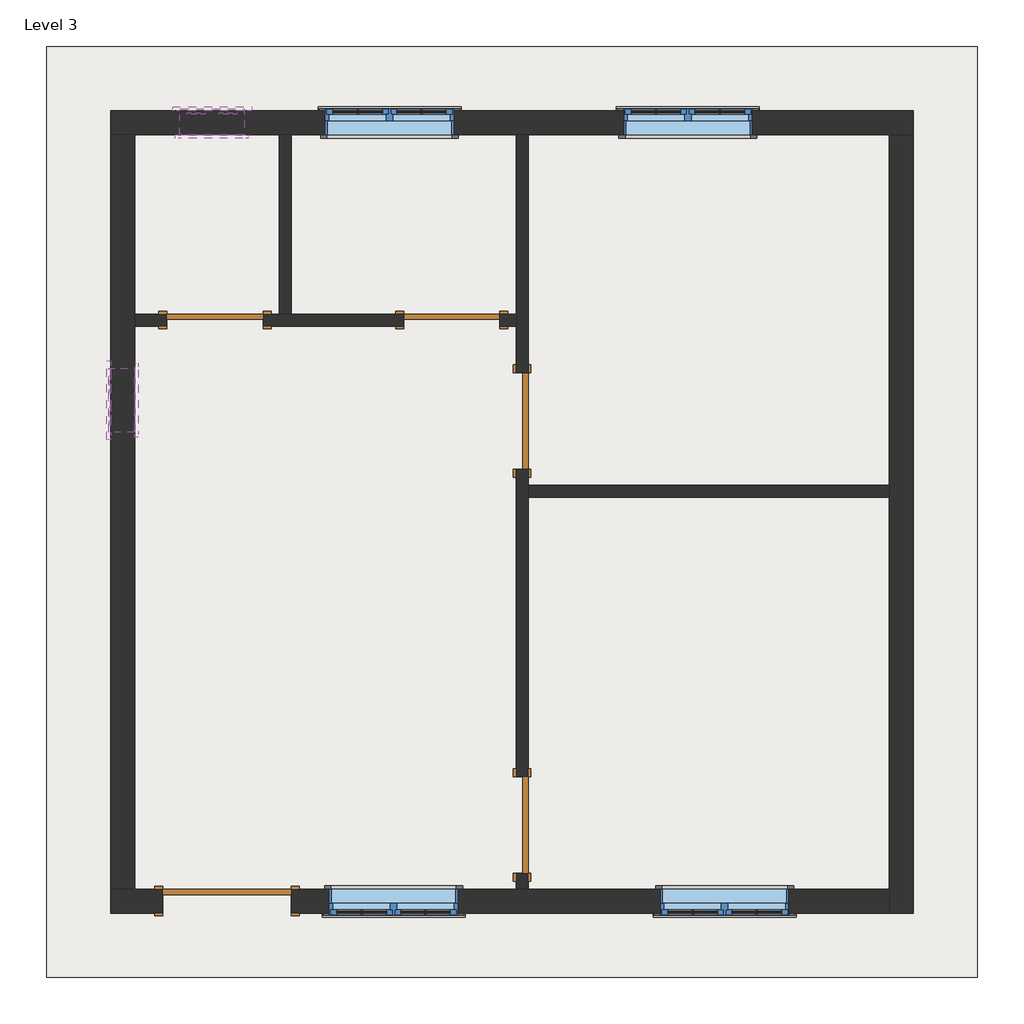
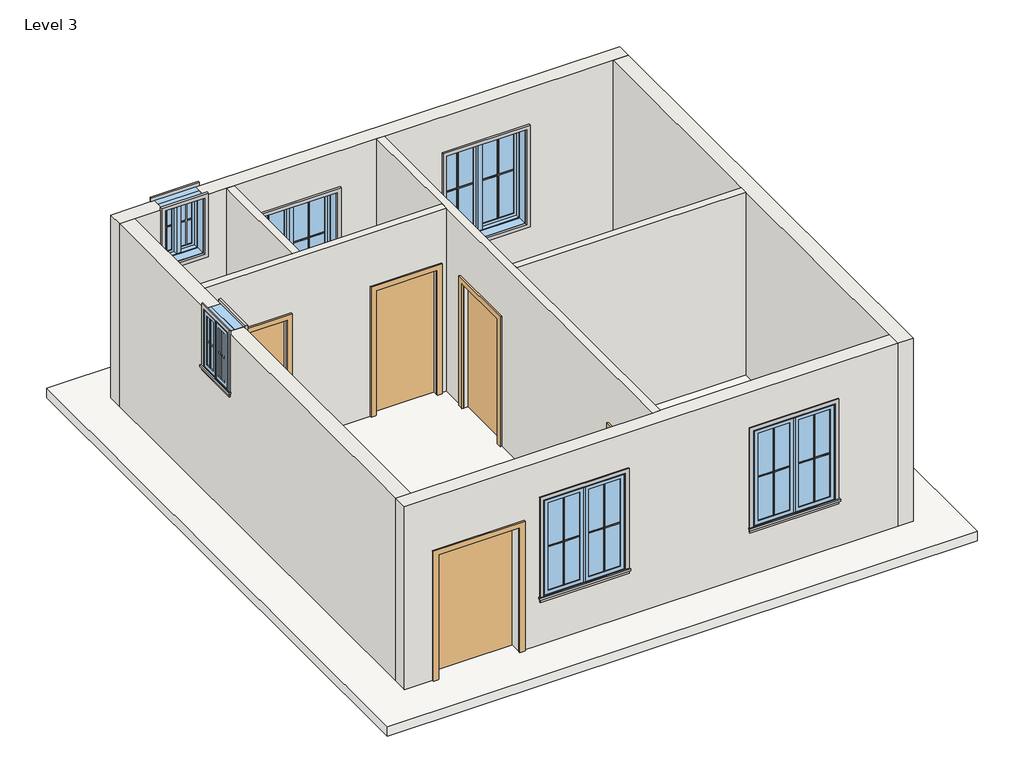
# One storey, incomplete: 24 proxies, 8 walls, 6 windows, 5 doors, 1 roof.
"""IFC4 building model written with IfcOpenShell, lengths in millimetres."""

from ifc_helpers import new_model, si_unit, frame, origin, place, context, project, spatial, polyline, outline, extrude, faceted_brep, transform, mapped, element, save
from components import muntin_pattern_2x2_muntin_pattern_2x2_6dad3731, muntin_pattern_2x2_muntin_pattern_2x2_a30a3345, muntin_pattern_2x2_muntin_pattern_2x2_53152e2c, muntin_pattern_2x2_muntin_pattern_2x2_e8f3e573, trim_window_exterior_flat_with_sill_92b9b949, trim_window_exterior_flat_with_sill_a665a915, trim_window_interior_flat_picture_frame_3bb882cf, trim_window_interior_flat_picture_frame_d485c387, door_e5f9f3c4, door_f4c4cdf2, window_c417fced, window_8377141f

model = new_model("IFC4")

# Units and contexts
model_context = context("Model", 3, world=origin())
ifc_project = project(units=[si_unit("LENGTHUNIT", "METRE", prefix="MILLI")], contexts=[model_context])

# Site, building, storey
site = spatial("IfcSite", under=ifc_project)
building = spatial("IfcBuilding", under=site)
storey = spatial("IfcBuildingStorey", under=building, Name="Level 3", Elevation=6096.0)

# Proxies
placement = place(None, origin())
muntin_pattern_2x2_muntin_pattern_2x2_shape = muntin_pattern_2x2_muntin_pattern_2x2_6dad3731(model_context)
element("IfcBuildingElementProxy", 1, Name="Muntin Pattern_2x2 : Muntin Pattern_2x2", ObjectType="Muntin Pattern_2x2 : Muntin Pattern_2x2", at=placement, inside=storey, context=model_context, shape_type="MappedRepresentation", body=[
    mapped(muntin_pattern_2x2_muntin_pattern_2x2_shape, transform((6192.8375, 13960.475, 7080.25), x_axis=(1.0, 0.0, 0.0), y_axis=(0.0, 1.0, 0.0), z_axis=(0.0, 0.0, 1.0))),
])
element("IfcBuildingElementProxy", 2, Name="Muntin Pattern_2x2 : Muntin Pattern_2x2", ObjectType="Muntin Pattern_2x2 : Muntin Pattern_2x2", at=placement, inside=storey, context=model_context, shape_type="MappedRepresentation", body=[
    mapped(muntin_pattern_2x2_muntin_pattern_2x2_shape, transform((7148.5125, 6359.525, 7080.25), x_axis=(-1.0, 0.0, 0.0), y_axis=(0.0, -1.0, 0.0), z_axis=(0.0, 0.0, 1.0))),
])
element("IfcBuildingElementProxy", 3, Name="Muntin Pattern_2x2 : Muntin Pattern_2x2", ObjectType="Muntin Pattern_2x2 : Muntin Pattern_2x2", at=placement, inside=storey, context=model_context, shape_type="MappedRepresentation", body=[
    mapped(muntin_pattern_2x2_muntin_pattern_2x2_shape, transform((4005.2625, 6359.525, 7080.25), x_axis=(-1.0, 0.0, 0.0), y_axis=(0.0, -1.0, 0.0), z_axis=(0.0, 0.0, 1.0))),
])
element("IfcBuildingElementProxy", 4, Name="Muntin Pattern_2x2 : Muntin Pattern_2x2", ObjectType="Muntin Pattern_2x2 : Muntin Pattern_2x2", at=placement, inside=storey, context=model_context, shape_type="MappedRepresentation", body=[
    mapped(muntin_pattern_2x2_muntin_pattern_2x2_shape, transform((3360.7375, 13960.475, 7080.25), x_axis=(1.0, 0.0, 0.0), y_axis=(0.0, 1.0, 0.0), z_axis=(0.0, 0.0, 1.0))),
])
muntin_pattern_2x2_muntin_pattern_2x2_2_shape = muntin_pattern_2x2_muntin_pattern_2x2_a30a3345(model_context)
element("IfcBuildingElementProxy", 5, Name="Muntin Pattern_2x2 : Muntin Pattern_2x2", ObjectType="Muntin Pattern_2x2 : Muntin Pattern_2x2", at=placement, inside=storey, context=model_context, shape_type="MappedRepresentation", body=[
    mapped(muntin_pattern_2x2_muntin_pattern_2x2_2_shape, transform((6799.2625, 13960.475, 7080.25), x_axis=(-1.0, 0.0, 0.0), y_axis=(0.0, -1.0, 0.0), z_axis=(0.0, 0.0, 1.0))),
])
element("IfcBuildingElementProxy", 6, Name="Muntin Pattern_2x2 : Muntin Pattern_2x2", ObjectType="Muntin Pattern_2x2 : Muntin Pattern_2x2", at=placement, inside=storey, context=model_context, shape_type="MappedRepresentation", body=[
    mapped(muntin_pattern_2x2_muntin_pattern_2x2_2_shape, transform((6542.0875, 6359.525, 7080.25), x_axis=(1.0, 0.0, 0.0), y_axis=(0.0, 1.0, 0.0), z_axis=(0.0, 0.0, 1.0))),
])
element("IfcBuildingElementProxy", 7, Name="Muntin Pattern_2x2 : Muntin Pattern_2x2", ObjectType="Muntin Pattern_2x2 : Muntin Pattern_2x2", at=placement, inside=storey, context=model_context, shape_type="MappedRepresentation", body=[
    mapped(muntin_pattern_2x2_muntin_pattern_2x2_2_shape, transform((3398.8375, 6359.525, 7080.25), x_axis=(1.0, 0.0, 0.0), y_axis=(0.0, 1.0, 0.0), z_axis=(0.0, 0.0, 1.0))),
])
element("IfcBuildingElementProxy", 8, Name="Muntin Pattern_2x2 : Muntin Pattern_2x2", ObjectType="Muntin Pattern_2x2 : Muntin Pattern_2x2", at=placement, inside=storey, context=model_context, shape_type="MappedRepresentation", body=[
    mapped(muntin_pattern_2x2_muntin_pattern_2x2_2_shape, transform((3967.1625, 13960.475, 7080.25), x_axis=(-1.0, 0.0, 0.0), y_axis=(0.0, -1.0, 0.0), z_axis=(0.0, 0.0, 1.0))),
])
muntin_pattern_2x2_muntin_pattern_2x2_3_shape = muntin_pattern_2x2_muntin_pattern_2x2_53152e2c(model_context)
element("IfcBuildingElementProxy", 9, Name="Muntin Pattern_2x2 : Muntin Pattern_2x2", ObjectType="Muntin Pattern_2x2 : Muntin Pattern_2x2", at=placement, inside=storey, context=model_context, shape_type="MappedRepresentation", body=[
    mapped(muntin_pattern_2x2_muntin_pattern_2x2_3_shape, transform((1025.525, 11069.6375, 8299.45), x_axis=(0.0, 1.0, 0.0), y_axis=(-1.0, 0.0, 0.0), z_axis=(0.0, 0.0, 1.0))),
])
element("IfcBuildingElementProxy", 10, Name="Muntin Pattern_2x2 : Muntin Pattern_2x2", ObjectType="Muntin Pattern_2x2 : Muntin Pattern_2x2", at=placement, inside=storey, context=model_context, shape_type="MappedRepresentation", body=[
    mapped(muntin_pattern_2x2_muntin_pattern_2x2_3_shape, transform((1827.2125, 13960.475, 8299.45), x_axis=(1.0, 0.0, 0.0), y_axis=(0.0, 1.0, 0.0), z_axis=(0.0, 0.0, 1.0))),
])
muntin_pattern_2x2_muntin_pattern_2x2_4_shape = muntin_pattern_2x2_muntin_pattern_2x2_e8f3e573(model_context)
element("IfcBuildingElementProxy", 11, Name="Muntin Pattern_2x2 : Muntin Pattern_2x2", ObjectType="Muntin Pattern_2x2 : Muntin Pattern_2x2", at=placement, inside=storey, context=model_context, shape_type="MappedRepresentation", body=[
    mapped(muntin_pattern_2x2_muntin_pattern_2x2_4_shape, transform((1025.525, 11371.2625, 8299.45), x_axis=(0.0, -1.0, 0.0), y_axis=(1.0, 0.0, 0.0), z_axis=(0.0, 0.0, 1.0))),
])
element("IfcBuildingElementProxy", 12, Name="Muntin Pattern_2x2 : Muntin Pattern_2x2", ObjectType="Muntin Pattern_2x2 : Muntin Pattern_2x2", at=placement, inside=storey, context=model_context, shape_type="MappedRepresentation", body=[
    mapped(muntin_pattern_2x2_muntin_pattern_2x2_4_shape, transform((2128.8375, 13960.475, 8299.45), x_axis=(-1.0, 0.0, 0.0), y_axis=(0.0, -1.0, 0.0), z_axis=(0.0, 0.0, 1.0))),
])
trim_window_exterior_flat_with_sill_shape = trim_window_exterior_flat_with_sill_92b9b949(model_context)
element("IfcBuildingElementProxy", 13, Name="Trim-Window-Exterior-Flat : with Sill", ObjectType="Trim-Window-Exterior-Flat : with Sill", at=placement, inside=storey, context=model_context, shape_type="MappedRepresentation", body=[
    mapped(trim_window_exterior_flat_with_sill_shape, transform((6496.05, 13970.0, 8534.4), x_axis=(-1.0, 0.0, 0.0), y_axis=(0.0, 0.0, 1.0), z_axis=(0.0, 1.0, 0.0))),
])
element("IfcBuildingElementProxy", 14, Name="Trim-Window-Exterior-Flat : with Sill", ObjectType="Trim-Window-Exterior-Flat : with Sill", at=placement, inside=storey, context=model_context, shape_type="MappedRepresentation", body=[
    mapped(trim_window_exterior_flat_with_sill_shape, transform((6845.3, 6350.0, 8534.4), x_axis=(1.0, 0.0, 0.0), y_axis=(0.0, 0.0, 1.0), z_axis=(0.0, -1.0, 0.0))),
])
element("IfcBuildingElementProxy", 15, Name="Trim-Window-Exterior-Flat : with Sill", ObjectType="Trim-Window-Exterior-Flat : with Sill", at=placement, inside=storey, context=model_context, shape_type="MappedRepresentation", body=[
    mapped(trim_window_exterior_flat_with_sill_shape, transform((3702.05, 6350.0, 8534.4), x_axis=(1.0, 0.0, 0.0), y_axis=(0.0, 0.0, 1.0), z_axis=(0.0, -1.0, 0.0))),
])
element("IfcBuildingElementProxy", 16, Name="Trim-Window-Exterior-Flat : with Sill", ObjectType="Trim-Window-Exterior-Flat : with Sill", at=placement, inside=storey, context=model_context, shape_type="MappedRepresentation", body=[
    mapped(trim_window_exterior_flat_with_sill_shape, transform((3663.95, 13970.0, 8534.4), x_axis=(-1.0, 0.0, 0.0), y_axis=(0.0, 0.0, 1.0), z_axis=(0.0, 1.0, 0.0))),
])
trim_window_exterior_flat_with_sill_2_shape = trim_window_exterior_flat_with_sill_a665a915(model_context)
element("IfcBuildingElementProxy", 17, Name="Trim-Window-Exterior-Flat : with Sill", ObjectType="Trim-Window-Exterior-Flat : with Sill", at=placement, inside=storey, context=model_context, shape_type="MappedRepresentation", body=[
    mapped(trim_window_exterior_flat_with_sill_2_shape, transform((1016.0, 11220.45, 9144.0), x_axis=(0.0, -1.0, 0.0), y_axis=(0.0, 0.0, 1.0), z_axis=(-1.0, 0.0, 0.0))),
])
element("IfcBuildingElementProxy", 18, Name="Trim-Window-Exterior-Flat : with Sill", ObjectType="Trim-Window-Exterior-Flat : with Sill", at=placement, inside=storey, context=model_context, shape_type="MappedRepresentation", body=[
    mapped(trim_window_exterior_flat_with_sill_2_shape, transform((1978.025, 13970.0, 9144.0), x_axis=(-1.0, 0.0, 0.0), y_axis=(0.0, 0.0, 1.0), z_axis=(0.0, 1.0, 0.0))),
])
trim_window_interior_flat_picture_frame_shape = trim_window_interior_flat_picture_frame_3bb882cf(model_context)
element("IfcBuildingElementProxy", 19, Name="Trim-Window-Interior-Flat : Picture Frame", ObjectType="Trim-Window-Interior-Flat : Picture Frame", at=placement, inside=storey, context=model_context, shape_type="MappedRepresentation", body=[
    mapped(trim_window_interior_flat_picture_frame_shape, transform((6496.05, 13741.4, 8534.4), x_axis=(1.0, 0.0, 0.0), y_axis=(0.0, 0.0, 1.0), z_axis=(0.0, -1.0, 0.0))),
])
element("IfcBuildingElementProxy", 20, Name="Trim-Window-Interior-Flat : Picture Frame", ObjectType="Trim-Window-Interior-Flat : Picture Frame", at=placement, inside=storey, context=model_context, shape_type="MappedRepresentation", body=[
    mapped(trim_window_interior_flat_picture_frame_shape, transform((6845.3, 6578.6, 8534.4), x_axis=(-1.0, 0.0, 0.0), y_axis=(0.0, 0.0, 1.0), z_axis=(0.0, 1.0, 0.0))),
])
element("IfcBuildingElementProxy", 21, Name="Trim-Window-Interior-Flat : Picture Frame", ObjectType="Trim-Window-Interior-Flat : Picture Frame", at=placement, inside=storey, context=model_context, shape_type="MappedRepresentation", body=[
    mapped(trim_window_interior_flat_picture_frame_shape, transform((3702.05, 6578.6, 8534.4), x_axis=(-1.0, 0.0, 0.0), y_axis=(0.0, 0.0, 1.0), z_axis=(0.0, 1.0, 0.0))),
])
element("IfcBuildingElementProxy", 22, Name="Trim-Window-Interior-Flat : Picture Frame", ObjectType="Trim-Window-Interior-Flat : Picture Frame", at=placement, inside=storey, context=model_context, shape_type="MappedRepresentation", body=[
    mapped(trim_window_interior_flat_picture_frame_shape, transform((3663.95, 13741.4, 8534.4), x_axis=(1.0, 0.0, 0.0), y_axis=(0.0, 0.0, 1.0), z_axis=(0.0, -1.0, 0.0))),
])
trim_window_interior_flat_picture_frame_2_shape = trim_window_interior_flat_picture_frame_d485c387(model_context)
element("IfcBuildingElementProxy", 23, Name="Trim-Window-Interior-Flat : Picture Frame", ObjectType="Trim-Window-Interior-Flat : Picture Frame", at=placement, inside=storey, context=model_context, shape_type="MappedRepresentation", body=[
    mapped(trim_window_interior_flat_picture_frame_2_shape, transform((1244.6, 11220.45, 9144.0), x_axis=(0.0, 1.0, 0.0), y_axis=(0.0, 0.0, 1.0), z_axis=(1.0, 0.0, 0.0))),
])
element("IfcBuildingElementProxy", 24, Name="Trim-Window-Interior-Flat : Picture Frame", ObjectType="Trim-Window-Interior-Flat : Picture Frame", at=placement, inside=storey, context=model_context, shape_type="MappedRepresentation", body=[
    mapped(trim_window_interior_flat_picture_frame_2_shape, transform((1978.025, 13741.4, 9144.0), x_axis=(1.0, 0.0, 0.0), y_axis=(0.0, 0.0, 1.0), z_axis=(0.0, -1.0, 0.0))),
])

# Doors
door_shape = door_e5f9f3c4(model_context)
element("IfcDoor", 25, ObjectType="Single-Flush : 36\" x 84\"", at=placement, inside=storey, context=model_context, shape_type="MappedRepresentation", body=[
    mapped(door_shape, transform((2006.6, 11982.45, 6096.0), x_axis=(1.0, 0.0, 0.0), y_axis=(0.0, 1.0, 0.0), z_axis=(0.0, 0.0, 1.0))),
])
element("IfcDoor", 26, ObjectType="Single-Flush : 36\" x 84\"", at=placement, inside=storey, context=model_context, shape_type="MappedRepresentation", body=[
    mapped(door_shape, transform((4254.5, 11982.45, 6096.0), x_axis=(1.0, 0.0, 0.0), y_axis=(0.0, 1.0, 0.0), z_axis=(0.0, 0.0, 1.0))),
])
element("IfcDoor", 27, ObjectType="Single-Flush : 36\" x 84\"", at=placement, inside=storey, context=model_context, shape_type="MappedRepresentation", body=[
    mapped(door_shape, transform((4921.25, 11023.6, 6096.0), x_axis=(0.0, -1.0, 0.0), y_axis=(1.0, 0.0, 0.0), z_axis=(0.0, 0.0, 1.0))),
])
element("IfcDoor", 28, ObjectType="Single-Flush : 36\" x 84\"", at=placement, inside=storey, context=model_context, shape_type="MappedRepresentation", body=[
    mapped(door_shape, transform((4921.25, 7188.2, 6096.0), x_axis=(0.0, -1.0, 0.0), y_axis=(1.0, 0.0, 0.0), z_axis=(0.0, 0.0, 1.0))),
])
door_2_shape = door_f4c4cdf2(model_context)
element("IfcDoor", 29, ObjectType="Single-Flush : 48\" x 84\"", at=placement, inside=storey, context=model_context, shape_type="MappedRepresentation", body=[
    mapped(door_2_shape, transform((2120.9, 6464.3, 6096.0), x_axis=(-1.0, 0.0, 0.0), y_axis=(0.0, -1.0, 0.0), z_axis=(0.0, 0.0, 1.0))),
])

# Roof
element("IfcRoof", 30, ObjectType="Generic - 12\"", at=placement, inside=storey, context=model_context, shape_type="SweptSolid", body=[
    extrude(outline(polyline([(406.4, 14579.6), (9245.6, 14579.6), (9245.6, 5740.4), (406.4, 5740.4), (406.4, 14579.6)])), frame((0.0, 0.0, 6096.0), z_axis=(0.0, 0.0, 1.0), x_axis=(1.0, 0.0, 0.0)), (0.0, 0.0, 1.0), 152.4),
])

# Walls
element("IfcWall", 31, ObjectType="Generic - 5\"", at=placement, inside=storey, context=model_context, shape_type="SweptSolid", body=[
    extrude(outline(polyline([(2616.2, 12039.6), (2616.2, 13741.4), (2730.5, 13741.4), (2730.5, 12039.6), (2616.2, 12039.6)])), frame((0.0, 0.0, 6096.0), z_axis=(0.0, 0.0, 1.0), x_axis=(1.0, 0.0, 0.0)), (0.0, 0.0, 1.0), 3048.0),
])
element("IfcWall", 32, ObjectType="Generic - 5\"", at=placement, inside=storey, context=model_context, shape_type="Brep", body=[
    faceted_brep([(4711.7, 11925.3, 8229.6), (4711.7, 11925.3, 6096.0), (4864.1, 11925.3, 6096.0), (4864.1, 11925.3, 9144.0), (1244.6, 11925.3, 9144.0), (1244.6, 11925.3, 6096.0), (1549.4, 11925.3, 6096.0), (1549.4, 11925.3, 8229.6), (2463.8, 11925.3, 8229.6), (2463.8, 11925.3, 6096.0), (3797.3, 11925.3, 6096.0), (3797.3, 11925.3, 8229.6), (4864.1, 12039.6, 6096.0), (4711.7, 12039.6, 6096.0), (4711.7, 12039.6, 8229.6), (3797.3, 12039.6, 8229.6), (3797.3, 12039.6, 6096.0), (2730.5, 12039.6, 6096.0), (2616.2, 12039.6, 6096.0), (2463.8, 12039.6, 6096.0), (2463.8, 12039.6, 8229.6), (1549.4, 12039.6, 8229.6), (1549.4, 12039.6, 6096.0), (1244.6, 12039.6, 6096.0), (1244.6, 12039.6, 9144.0), (2616.2, 12039.6, 9144.0), (2730.5, 12039.6, 9144.0), (4864.1, 12039.6, 9144.0)], [[[0, 1, 2, 3, 4, 5, 6, 7, 8, 9, 10, 11]], [[12, 13, 14, 15, 16, 17, 18, 19, 20, 21, 22, 23, 24, 25, 26, 27]], [[6, 5, 23, 22]], [[10, 9, 19, 18, 17, 16]], [[2, 1, 13, 12]], [[4, 3, 27, 26, 25, 24]], [[5, 4, 24, 23]], [[3, 2, 12, 27]], [[20, 19, 9, 8]], [[21, 20, 8, 7]], [[22, 21, 7, 6]], [[14, 13, 1, 0]], [[15, 14, 0, 11]], [[16, 15, 11, 10]]]),
])
element("IfcWall", 33, ObjectType="Generic - 5\"", at=placement, inside=storey, context=model_context, shape_type="Brep", body=[
    faceted_brep([(4864.1, 6731.0, 8229.6), (4864.1, 6731.0, 6096.0), (4864.1, 6578.6, 6096.0), (4864.1, 6578.6, 9144.0), (4864.1, 11925.3, 9144.0), (4864.1, 12039.6, 9144.0), (4864.1, 13741.4, 9144.0), (4864.1, 13741.4, 6096.0), (4864.1, 12039.6, 6096.0), (4864.1, 11925.3, 6096.0), (4864.1, 11480.8, 6096.0), (4864.1, 11480.8, 8229.6), (4864.1, 10566.4, 8229.6), (4864.1, 10566.4, 6096.0), (4864.1, 7645.4, 6096.0), (4864.1, 7645.4, 8229.6), (4978.4, 6578.6, 6096.0), (4978.4, 6731.0, 6096.0), (4978.4, 6731.0, 8229.6), (4978.4, 7645.4, 8229.6), (4978.4, 7645.4, 6096.0), (4978.4, 10299.7, 6096.0), (4978.4, 10414.0, 6096.0), (4978.4, 10566.4, 6096.0), (4978.4, 10566.4, 8229.6), (4978.4, 11480.8, 8229.6), (4978.4, 11480.8, 6096.0), (4978.4, 13741.4, 6096.0), (4978.4, 13741.4, 9144.0), (4978.4, 10414.0, 9144.0), (4978.4, 10299.7, 9144.0), (4978.4, 6578.6, 9144.0)], [[[0, 1, 2, 3, 4, 5, 6, 7, 8, 9, 10, 11, 12, 13, 14, 15]], [[16, 17, 18, 19, 20, 21, 22, 23, 24, 25, 26, 27, 28, 29, 30, 31]], [[10, 9, 8, 7, 27, 26]], [[14, 13, 23, 22, 21, 20]], [[2, 1, 17, 16]], [[6, 5, 4, 3, 31, 30, 29, 28]], [[7, 6, 28, 27]], [[3, 2, 16, 31]], [[24, 23, 13, 12]], [[25, 24, 12, 11]], [[26, 25, 11, 10]], [[18, 17, 1, 0]], [[19, 18, 0, 15]], [[20, 19, 15, 14]]]),
])
element("IfcWall", 34, ObjectType="Generic - 5\"", at=placement, inside=storey, context=model_context, shape_type="SweptSolid", body=[
    extrude(outline(polyline([(8407.4, 10299.7), (4978.4, 10299.7), (4978.4, 10414.0), (8407.4, 10414.0), (8407.4, 10299.7)])), frame((0.0, 0.0, 6096.0), z_axis=(0.0, 0.0, 1.0), x_axis=(1.0, 0.0, 0.0)), (0.0, 0.0, 1.0), 3048.0),
])
element("IfcWall", 35, ObjectType="Generic - 8\"", at=placement, inside=storey, context=model_context, shape_type="Brep", body=[
    faceted_brep([(1016.0, 13741.4, 6096.0), (1244.6, 13741.4, 6096.0), (2616.2, 13741.4, 6096.0), (2730.5, 13741.4, 6096.0), (4864.1, 13741.4, 6096.0), (4978.4, 13741.4, 6096.0), (8407.4, 13741.4, 6096.0), (8636.0, 13741.4, 6096.0), (8636.0, 13741.4, 9144.0), (8407.4, 13741.4, 9144.0), (4978.4, 13741.4, 9144.0), (4864.1, 13741.4, 9144.0), (2730.5, 13741.4, 9144.0), (2616.2, 13741.4, 9144.0), (2282.825, 13741.4, 9144.0), (2282.825, 13741.4, 8229.6), (1673.225, 13741.4, 8229.6), (1673.225, 13741.4, 9144.0), (1244.6, 13741.4, 9144.0), (1016.0, 13741.4, 9144.0), (7105.65, 13741.4, 8534.4), (7105.65, 13741.4, 7010.4), (5886.45, 13741.4, 7010.4), (5886.45, 13741.4, 8534.4), (4273.55, 13741.4, 8534.4), (4273.55, 13741.4, 7010.4), (3054.35, 13741.4, 7010.4), (3054.35, 13741.4, 8534.4), (8636.0, 13970.0, 6096.0), (1016.0, 13970.0, 6096.0), (1016.0, 13970.0, 9144.0), (1673.225, 13970.0, 9144.0), (1673.225, 13970.0, 8229.6), (2282.825, 13970.0, 8229.6), (2282.825, 13970.0, 9144.0), (8636.0, 13970.0, 9144.0), (7105.65, 13970.0, 7010.4), (7105.65, 13970.0, 8534.4), (5886.45, 13970.0, 8534.4), (5886.45, 13970.0, 7010.4), (4273.55, 13970.0, 7010.4), (4273.55, 13970.0, 8534.4), (3054.35, 13970.0, 8534.4), (3054.35, 13970.0, 7010.4)], [[[0, 1, 2, 3, 4, 5, 6, 7, 8, 9, 10, 11, 12, 13, 14, 15, 16, 17, 18, 19], [20, 21, 22, 23], [24, 25, 26, 27]], [[28, 29, 30, 31, 32, 33, 34, 35], [36, 37, 38, 39], [40, 41, 42, 43]], [[7, 6, 5, 4, 3, 2, 1, 0, 29, 28]], [[8, 35, 34, 14, 13, 12, 11, 10, 9]], [[30, 19, 18, 17, 31]], [[8, 7, 28, 35]], [[0, 19, 30, 29]], [[21, 20, 37, 36]], [[22, 21, 36, 39]], [[23, 22, 39, 38]], [[20, 23, 38, 37]], [[25, 24, 41, 40]], [[26, 25, 40, 43]], [[27, 26, 43, 42]], [[24, 27, 42, 41]], [[33, 15, 14, 34]], [[15, 33, 32, 16]], [[16, 32, 31, 17]]]),
])
element("IfcWall", 36, ObjectType="Generic - 8\"", at=placement, inside=storey, context=model_context, shape_type="Brep", body=[
    faceted_brep([(8407.4, 13741.4, 6096.0), (8407.4, 10414.0, 6096.0), (8407.4, 10299.7, 6096.0), (8407.4, 6578.6, 6096.0), (8407.4, 6350.0, 6096.0), (8407.4, 6350.0, 9144.0), (8407.4, 6578.6, 9144.0), (8407.4, 10299.7, 9144.0), (8407.4, 10414.0, 9144.0), (8407.4, 13741.4, 9144.0), (8636.0, 13741.4, 6096.0), (8636.0, 13741.4, 9144.0), (8636.0, 6350.0, 9144.0), (8636.0, 6350.0, 6096.0)], [[[0, 1, 2, 3, 4, 5, 6, 7, 8, 9]], [[10, 11, 12, 13]], [[4, 3, 2, 1, 0, 10, 13]], [[9, 8, 7, 6, 5, 12, 11]], [[0, 9, 11, 10]], [[5, 4, 13, 12]]]),
])
element("IfcWall", 37, ObjectType="Generic - 8\"", at=placement, inside=storey, context=model_context, shape_type="Brep", body=[
    faceted_brep([(1511.3, 6578.6, 8229.6), (1511.3, 6578.6, 6096.0), (1244.6, 6578.6, 6096.0), (1016.0, 6578.6, 6096.0), (1016.0, 6578.6, 9144.0), (1244.6, 6578.6, 9144.0), (4864.1, 6578.6, 9144.0), (4978.4, 6578.6, 9144.0), (8407.4, 6578.6, 9144.0), (8407.4, 6578.6, 6096.0), (4978.4, 6578.6, 6096.0), (4864.1, 6578.6, 6096.0), (2730.5, 6578.6, 6096.0), (2730.5, 6578.6, 8229.6), (6235.7, 6578.6, 8534.4), (6235.7, 6578.6, 7010.4), (7454.9, 6578.6, 7010.4), (7454.9, 6578.6, 8534.4), (3092.45, 6578.6, 8534.4), (3092.45, 6578.6, 7010.4), (4311.65, 6578.6, 7010.4), (4311.65, 6578.6, 8534.4), (1016.0, 6350.0, 6096.0), (1511.3, 6350.0, 6096.0), (1511.3, 6350.0, 8229.6), (2730.5, 6350.0, 8229.6), (2730.5, 6350.0, 6096.0), (8407.4, 6350.0, 6096.0), (8407.4, 6350.0, 9144.0), (1016.0, 6350.0, 9144.0), (6235.7, 6350.0, 8534.4), (7454.9, 6350.0, 8534.4), (7454.9, 6350.0, 7010.4), (6235.7, 6350.0, 7010.4), (3092.45, 6350.0, 8534.4), (4311.65, 6350.0, 8534.4), (4311.65, 6350.0, 7010.4), (3092.45, 6350.0, 7010.4)], [[[0, 1, 2, 3, 4, 5, 6, 7, 8, 9, 10, 11, 12, 13], [14, 15, 16, 17], [18, 19, 20, 21]], [[22, 23, 24, 25, 26, 27, 28, 29], [30, 31, 32, 33], [34, 35, 36, 37]], [[3, 2, 1, 23, 22]], [[12, 11, 10, 9, 27, 26]], [[8, 7, 6, 5, 4, 29, 28]], [[9, 8, 28, 27]], [[4, 3, 22, 29]], [[24, 23, 1, 0]], [[25, 24, 0, 13]], [[26, 25, 13, 12]], [[15, 14, 30, 33]], [[16, 15, 33, 32]], [[17, 16, 32, 31]], [[14, 17, 31, 30]], [[19, 18, 34, 37]], [[20, 19, 37, 36]], [[21, 20, 36, 35]], [[18, 21, 35, 34]]]),
])
element("IfcWall", 38, ObjectType="Generic - 8\"", at=placement, inside=storey, context=model_context, shape_type="Brep", body=[
    faceted_brep([(1244.6, 6578.6, 6096.0), (1244.6, 11925.3, 6096.0), (1244.6, 12039.6, 6096.0), (1244.6, 13741.4, 6096.0), (1244.6, 13741.4, 9144.0), (1244.6, 12039.6, 9144.0), (1244.6, 11925.3, 9144.0), (1244.6, 11525.25, 9144.0), (1244.6, 11525.25, 8229.6), (1244.6, 10915.65, 8229.6), (1244.6, 10915.65, 9144.0), (1244.6, 6578.6, 9144.0), (1016.0, 13741.4, 6096.0), (1016.0, 6578.6, 6096.0), (1016.0, 6578.6, 9144.0), (1016.0, 10915.65, 9144.0), (1016.0, 10915.65, 8229.6), (1016.0, 11525.25, 8229.6), (1016.0, 11525.25, 9144.0), (1016.0, 13741.4, 9144.0)], [[[0, 1, 2, 3, 4, 5, 6, 7, 8, 9, 10, 11]], [[12, 13, 14, 15, 16, 17, 18, 19]], [[3, 2, 1, 0, 13, 12]], [[14, 11, 10, 15]], [[4, 19, 18, 7, 6, 5]], [[4, 3, 12, 19]], [[0, 11, 14, 13]], [[17, 8, 7, 18]], [[8, 17, 16, 9]], [[9, 16, 15, 10]]]),
])

# Windows
window_shape = window_c417fced(model_context)
element("IfcWindow", 39, ObjectType="Window-Casement-Double : 24\" x 36\"", at=placement, inside=storey, context=model_context, shape_type="MappedRepresentation", body=[
    mapped(window_shape, transform((1130.3, 11220.45, 7315.2), x_axis=(0.0, 1.0, 0.0), y_axis=(-1.0, 0.0, 0.0), z_axis=(0.0, 0.0, 1.0))),
])
element("IfcWindow", 40, ObjectType="Window-Casement-Double : 24\" x 36\"", at=placement, inside=storey, context=model_context, shape_type="MappedRepresentation", body=[
    mapped(window_shape, transform((1978.025, 13855.7, 7315.2), x_axis=(1.0, 0.0, 0.0), y_axis=(0.0, 1.0, 0.0), z_axis=(0.0, 0.0, 1.0))),
])
window_2_shape = window_8377141f(model_context)
element("IfcWindow", 41, ObjectType="Window-Casement-Double : 48\" x 60\"", at=placement, inside=storey, context=model_context, shape_type="MappedRepresentation", body=[
    mapped(window_2_shape, transform((6496.05, 13855.7, 6096.0), x_axis=(1.0, 0.0, 0.0), y_axis=(0.0, 1.0, 0.0), z_axis=(0.0, 0.0, 1.0))),
])
element("IfcWindow", 42, ObjectType="Window-Casement-Double : 48\" x 60\"", at=placement, inside=storey, context=model_context, shape_type="MappedRepresentation", body=[
    mapped(window_2_shape, transform((6845.3, 6464.3, 6096.0), x_axis=(-1.0, 0.0, 0.0), y_axis=(0.0, -1.0, 0.0), z_axis=(0.0, 0.0, 1.0))),
])
element("IfcWindow", 43, ObjectType="Window-Casement-Double : 48\" x 60\"", at=placement, inside=storey, context=model_context, shape_type="MappedRepresentation", body=[
    mapped(window_2_shape, transform((3702.05, 6464.3, 6096.0), x_axis=(-1.0, 0.0, 0.0), y_axis=(0.0, -1.0, 0.0), z_axis=(0.0, 0.0, 1.0))),
])
element("IfcWindow", 44, ObjectType="Window-Casement-Double : 48\" x 60\"", at=placement, inside=storey, context=model_context, shape_type="MappedRepresentation", body=[
    mapped(window_2_shape, transform((3663.95, 13855.7, 6096.0), x_axis=(1.0, 0.0, 0.0), y_axis=(0.0, 1.0, 0.0), z_axis=(0.0, 0.0, 1.0))),
])

save(model, "model.ifc")

# Revit data of these elements
# Type "Muntin Pattern_2x2 : Muntin Pattern_2x2"
#   Width [instance default] = 4' - 0"
#   Thickness = 0' - 0 1/2"
#   Height [instance default] = 4' - 0"
#   Distance = 0' - 0 3/4"
#   Interior Material [instance default] = none
#   Exterior Material [instance default] = none
#   Default Elevation = 0
# Type "Trim-Window-Exterior-Flat : with Sill"
#   Trim Width = 0' - 2 1/4"
#   Trim Thickness_Picture Frame = 0' - 1 1/4"
#   Trim Thickness_with Sill = 0' - 0 3/4"
#   Sill Thickness = 0' - 1 1/4"
#   Opening Width [instance default] = 2' - 0"
#   Opening Height [instance default] = 3' - 0"
#   Default Elevation = 4' - 0"
#   Sill = yes
#   Picture Frame = no
#   Trim Material [instance default] = none
# Type "Trim-Window-Interior-Flat : Picture Frame"
#   Trim Thickness_Picture Frame = 0' - 1 1/4"
#   Trim Width = 0' - 2 1/4"
#   Trim Thickness_with Sill = 0' - 0 3/4"
#   Sill Thickness = 0' - 1 1/4"
#   Opening Width [instance default] = 2' - 0"
#   Opening Height [instance default] = 3' - 0"
#   Default Elevation = 4' - 0"
#   Sill = no
#   Picture Frame = yes
#   Trim Material [instance default] = none
# Type "Single-Flush : 36\" x 84\""
#   Type Mark = "1"
#   Construction Type Id = "MDOOR"
#   Assembly Code = "C1020"
#   Analytic Construction = "Metal"
#   Thickness = 0' - 2"
#   Heat Transfer Coefficient (U) = 0.651978 BTU/(h·ft²·°F)
#   Height = 7' - 0"
#   Trim Projection Ext = 0' - 1"
#   Trim Projection Int = 0' - 1"
#   Trim Width = 0' - 3"
#   Width = 3' - 0"
#   Define Thermal Properties by = 1
#   Define Thermal Properties by = 1
#   Door Material = Door - Panel
#   Frame Material = Door - Frame
#   Visual Light Transmittance = 0
#   Solar Heat Gain Coefficient = 0
#   Function = (empty or 0)
#   Wall Closure = (empty or 0)
# Type "Single-Flush : 48\" x 84\""
#   Type Mark = "5"
#   Construction Type Id = "MDOOR"
#   Assembly Code = "C1020"
#   Analytic Construction = "Metal"
#   Thickness = 0' - 2"
#   Heat Transfer Coefficient (U) = 0.651978 BTU/(h·ft²·°F)
#   Height = 7' - 0"
#   Trim Projection Ext = 0' - 1"
#   Trim Projection Int = 0' - 1"
#   Trim Width = 0' - 3"
#   Width = 4' - 0"
#   Define Thermal Properties by = 1
#   Define Thermal Properties by = 1
#   Door Material = Door - Panel
#   Frame Material = Door - Frame
#   Visual Light Transmittance = 0
#   Solar Heat Gain Coefficient = 0
#   Function = (empty or 0)
#   Wall Closure = (empty or 0)
# Type "Generic - 12\""
#   Assembly Code = "B1020"
#   Layers, outside or top first: 0' - 6" no material (function 1)
# Type "Generic - 5\""
#   Assembly Code = "B2010"
#   Layers, outside or top first: 0' - 4 1/2" no material (function 1)
# Type "Generic - 8\""
#   Assembly Code = "B2010"
#   Layers, outside or top first: 0' - 9" "Parking Stripe" (function 1)
# Type "Window-Casement-Double : 24\" x 36\""
#   Type Mark = "14"
#   Fire Rating = "0.5h"
#   Assembly Code = "B2020100"
#   Analytic Construction = "Double glazing - domestic"
#   Frame Extension [instance default] = 0' - 0 1/4"
#   Window Inset [instance default] = 0' - 0"
#   Wall Thickness [instance default] = 0' - 6"
#   Interior Wall Closure [instance default] = 0' - 2 1/4"
#   Half Width = 1' - 0"
#   Visual Light Transmittance = 0.81
#   Thermal Resistance (R) = 1.8146 (h·ft²·°F)/BTU
#   Solar Heat Gain Coefficient = 0.76
#   Rough Width = 2' - 0 1/2"
#   Rough Height = 3' - 0 1/2"
#   Height = 3' - 0"
#   Heat Transfer Coefficient (U) = 0.5511 BTU/(h·ft²·°F)
#   Exterior Wall Closure [instance default] = 0' - 1 1/4"
#   Extension Jamb [instance default] = 0' - 2 1/4"
#   Default Sill Height = 3' - 0"
#   Width = 2' - 0"
#   Define Thermal Properties by = 0
#   Muntin Visibility = yes
#   Interior Trim Visibility [instance default] = yes
#   Exterior Trim Visibility [instance default] = yes
#   Extension Jamb Visibility [instance default] = yes
#   Interior Trim Material = Wood - Stained
#   Muntin Pattern = Muntin Pattern_2x2 : Muntin Pattern_2x2
#   Interior Trim = Trim-Window-Interior-Flat : Picture Frame
#   Interior Frame Material = Wood - Stained
#   Glass Panel Material = Glass
#   Exterior Trim Material = Clad - White
#   Exterior Trim = Trim-Window-Exterior-Flat : with Sill
#   Exterior Frame Material = Clad - White
#   Wall Closure = (empty or 0)
# Type "Window-Casement-Double : 48\" x 60\""
#   Type Mark = "17"
#   Fire Rating = "0.5h"
#   Assembly Code = "B2020100"
#   Analytic Construction = "Double glazing - domestic"
#   Frame Extension [instance default] = 0' - 0 1/4"
#   Window Inset [instance default] = 0' - 0"
#   Wall Thickness [instance default] = 0' - 6"
#   Interior Wall Closure [instance default] = 0' - 2 1/4"
#   Half Width = 2' - 0"
#   Visual Light Transmittance = 0.81
#   Thermal Resistance (R) = 1.8146 (h·ft²·°F)/BTU
#   Solar Heat Gain Coefficient = 0.76
#   Rough Width = 4' - 0 1/2"
#   Rough Height = 5' - 0 1/2"
#   Height = 5' - 0"
#   Heat Transfer Coefficient (U) = 0.5511 BTU/(h·ft²·°F)
#   Exterior Wall Closure [instance default] = 0' - 1 1/4"
#   Extension Jamb [instance default] = 0' - 2 1/4"
#   Default Sill Height = 3' - 0"
#   Width = 4' - 0"
#   Define Thermal Properties by = 0
#   Muntin Visibility = yes
#   Interior Trim Visibility [instance default] = yes
#   Exterior Trim Visibility [instance default] = yes
#   Extension Jamb Visibility [instance default] = yes
#   Interior Trim Material = Wood - Stained
#   Muntin Pattern = Muntin Pattern_2x2 : Muntin Pattern_2x2
#   Interior Trim = Trim-Window-Interior-Flat : Picture Frame
#   Interior Frame Material = Wood - Stained
#   Glass Panel Material = Glass
#   Exterior Trim Material = Clad - White
#   Exterior Trim = Trim-Window-Exterior-Flat : with Sill
#   Exterior Frame Material = Clad - White
#   Wall Closure = (empty or 0)
# Elements 1, 2, 3, 4, 5, 6, 7, 8 (IfcBuildingElementProxy, "Muntin Pattern_2x2 : Muntin Pattern_2x2")
#   Width = 1' - 6 5/8"
#   Height = 4' - 6 1/2"
#   Interior Material = Wood - Stained
#   Exterior Material = Clad - White
#   Phase Created = New Construction
#   Materials on its faces: "Clad - White", "Wood - Stained"
# Elements 9, 10, 11, 12 (IfcBuildingElementProxy, "Muntin Pattern_2x2 : Muntin Pattern_2x2")
#   Width = 0' - 6 5/8"
#   Height = 2' - 6 1/2"
#   Interior Material = Wood - Stained
#   Exterior Material = Clad - White
#   Phase Created = New Construction
#   Materials on its faces: "Clad - White", "Wood - Stained"
# Elements 13, 14, 15, 16 (IfcBuildingElementProxy, "Trim-Window-Exterior-Flat : with Sill")
#   Opening Width = 4' - 0"
#   Opening Height = 5' - 0"
#   Trim Material = Clad - White
#   Phase Created = New Construction
#   Materials on its faces: "Clad - White"
# Elements 17, 18 (IfcBuildingElementProxy, "Trim-Window-Exterior-Flat : with Sill")
#   Opening Width = 2' - 0"
#   Opening Height = 3' - 0"
#   Trim Material = Clad - White
#   Phase Created = New Construction
#   Materials on its faces: "Clad - White"
# Elements 19, 20, 21, 22 (IfcBuildingElementProxy, "Trim-Window-Interior-Flat : Picture Frame")
#   Opening Width = 4' - 0"
#   Opening Height = 5' - 0"
#   Trim Material = Wood - Stained
#   Phase Created = New Construction
#   Materials on its faces: "Wood - Stained"
# Elements 23, 24 (IfcBuildingElementProxy, "Trim-Window-Interior-Flat : Picture Frame")
#   Opening Width = 2' - 0"
#   Opening Height = 3' - 0"
#   Trim Material = Wood - Stained
#   Phase Created = New Construction
#   Materials on its faces: "Wood - Stained"
# Elements 25, 26, 27, 28 (IfcDoor, "Single-Flush : 36\" x 84\"")
#   Phase Created = New Construction
#   Materials on its faces: "Door - Frame", "Door - Panel"
# Element 29 (IfcDoor, "Single-Flush : 48\" x 84\"")
#   Phase Created = New Construction
#   Materials on its faces: "Door - Frame", "Door - Panel"
# Element 30 (IfcRoof, "Generic - 12\"")
#   built-in parameter 1001705 = 20.5 (stored number, unit not read)
#   built-in parameter 1001710 = 33615
#   Phase Created = New Construction
#   Materials on its faces: "Textile - Linen, Smooth", "Default Roof"
# Elements 31, 32, 33, 34 (IfcWall, "Generic - 5\"")
#   Top Offset = 0' - 0"
#   Base Offset = 0' - 0"
#   wall height = 10' - 0"
#   Phase Created = New Construction
#   Base Constraint = Level 3
#   Top Constraint = Level 4
#   Materials on its faces: "Default Wall"
# Elements 35, 36, 37, 38 (IfcWall, "Generic - 8\"")
#   Top Offset = 0' - 0"
#   Base Offset = 0' - 0"
#   Unconnected Height = 10' - 0"
#   wall height = 10' - 0"
#   Phase Created = New Construction
#   Base Constraint = Level 3
#   Materials on its faces: "Parking Stripe", "Wood Planks"
# Element 39 (IfcWindow, "Window-Casement-Double : 24\" x 36\"")
#   Mark = "17"
#   Window Inset = 0' - 0"
#   Interior Wall Closure = 0' - 2 1/4"
#   Frame Extension = 0' - 0 1/4"
#   Exterior Wall Closure = 0' - 1 1/4"
#   Interior Trim Visibility = yes
#   Exterior Trim Visibility = yes
#   Phase Created = New Construction
#   Materials on its faces: "Wood - Stained", "Glass", "Clad - White"
# Element 40 (IfcWindow, "Window-Casement-Double : 24\" x 36\"")
#   Mark = "18"
#   Window Inset = 0' - 0"
#   Interior Wall Closure = 0' - 2 1/4"
#   Frame Extension = 0' - 0 1/4"
#   Exterior Wall Closure = 0' - 1 1/4"
#   Interior Trim Visibility = yes
#   Exterior Trim Visibility = yes
#   Phase Created = New Construction
#   Materials on its faces: "Wood - Stained", "Glass", "Clad - White"
# Element 41 (IfcWindow, "Window-Casement-Double : 48\" x 60\"")
#   Mark = "13"
#   Window Inset = 0' - 0"
#   Interior Wall Closure = 0' - 2 1/4"
#   Frame Extension = 0' - 0 1/4"
#   Exterior Wall Closure = 0' - 1 1/4"
#   Interior Trim Visibility = yes
#   Exterior Trim Visibility = yes
#   Phase Created = New Construction
#   Materials on its faces: "Wood - Stained", "Glass", "Clad - White"
# Element 42 (IfcWindow, "Window-Casement-Double : 48\" x 60\"")
#   Mark = "14"
#   Window Inset = 0' - 0"
#   Interior Wall Closure = 0' - 2 1/4"
#   Frame Extension = 0' - 0 1/4"
#   Exterior Wall Closure = 0' - 1 1/4"
#   Interior Trim Visibility = yes
#   Exterior Trim Visibility = yes
#   Phase Created = New Construction
#   Materials on its faces: "Wood - Stained", "Glass", "Clad - White"
# Element 43 (IfcWindow, "Window-Casement-Double : 48\" x 60\"")
#   Mark = "15"
#   Window Inset = 0' - 0"
#   Interior Wall Closure = 0' - 2 1/4"
#   Frame Extension = 0' - 0 1/4"
#   Exterior Wall Closure = 0' - 1 1/4"
#   Interior Trim Visibility = yes
#   Exterior Trim Visibility = yes
#   Phase Created = New Construction
#   Materials on its faces: "Wood - Stained", "Glass", "Clad - White"
# Element 44 (IfcWindow, "Window-Casement-Double : 48\" x 60\"")
#   Mark = "16"
#   Window Inset = 0' - 0"
#   Interior Wall Closure = 0' - 2 1/4"
#   Frame Extension = 0' - 0 1/4"
#   Exterior Wall Closure = 0' - 1 1/4"
#   Interior Trim Visibility = yes
#   Exterior Trim Visibility = yes
#   Phase Created = New Construction
#   Materials on its faces: "Wood - Stained", "Glass", "Clad - White"
# Materials
#   "Door - Panel": class "Wood", colour RGB 210 159 95, transparency 0, Cost = 0
#   "Door - Frame": colour RGB 118 70 51, transparency 0, Cost = 0
#   "Parking Stripe": class "Paint", colour RGB 250 250 91, transparency 0, Cost = 0
#   "Wood - Stained": class "Wood", colour RGB 224 178 126, transparency 0, Cost = 0
#   "Glass": class "Glass", colour RGB 0 128 192, transparency 0.75, Description = "Soda Lime Glass", Cost = 0
#   "Clad - White": class "Wood", colour RGB 242 242 238, transparency 0, Cost = 0
#   "Textile - Linen, Smooth": colour RGB 249 239 230, transparency 0
#   "Default Roof": colour RGB 88 101 114, transparency 0, Cost = 0
#   "Default Wall": colour RGB 128 128 128, transparency 0, Cost = 0
#   "Wood Planks": class "Wood", colour RGB 193 160 115, transparency 0, Description = "Physical material.", Cost = 0
